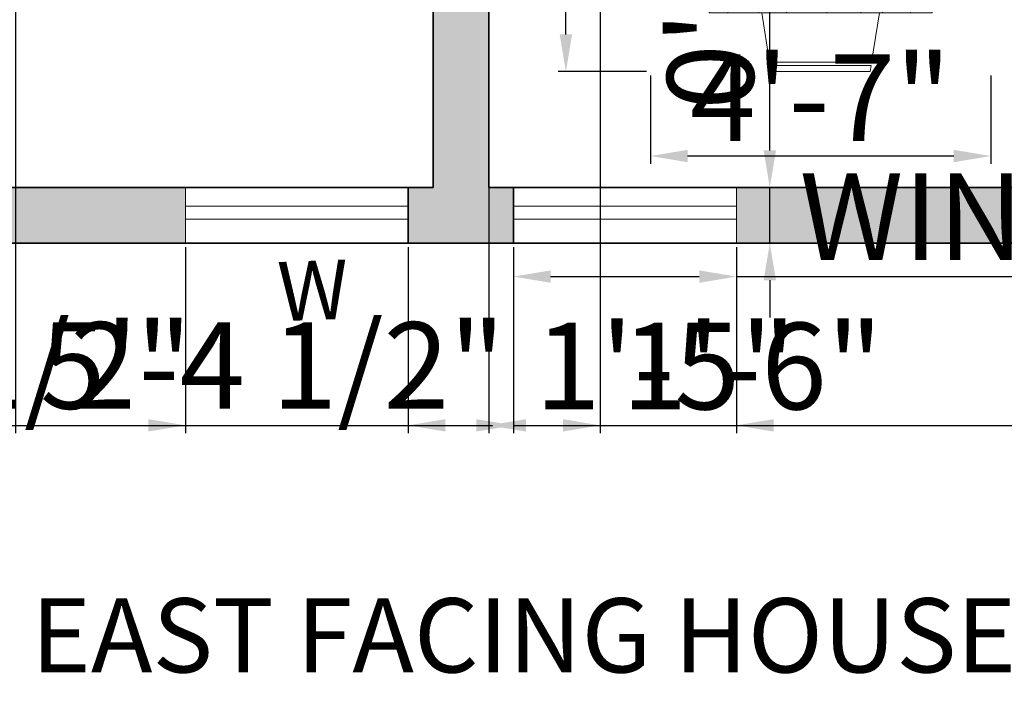
# Model space of a CAD drawing. Units: inches. Extents: x 2961 to 3748, y 1432 to 1961.
# Tile 2 of 9: x 3188 to 3348, y 1432 to 1541. Entities that reach past the tile are written whole.
import ezdxf
from ezdxf.enums import TextEntityAlignment as Align

# ---------------------------------------------------------------- set-up
doc = ezdxf.new("R2010")
doc.units = ezdxf.units.IN
for name, color, linetype, lineweight in [('A-ANNO-DIMS', 2, 'Continuous', 18), ('A-ANNO-TEXT', 7, 'Continuous', 18), ('A-ANNO-TITL', 7, 'Continuous', 25), ('A-FURN', 8, 'Continuous', 18), ('A-GLAZ', 4, 'Continuous', 18), ('A-WALL', 7, 'Continuous', 35), ('A-WALL-PATT', 252, 'Continuous', 13)]:
    doc.layers.add(name, color=color, linetype=linetype, lineweight=lineweight)
doc.styles.get("Standard").update_dxf_attribs({"font": 'arial.ttf'})
doc.dimstyles.new('ISO-25', dxfattribs={"dimtxt": 14, "dimasz": 6, "dimexe": 1.25, "dimexo": 0.625, "dimtad": 1, "dimlunit": 3, "dimtxsty": 'Standard', "dimcen": 2.5, "dimadec": 0, "dimazin": 0, "dimtfac": 1, "dimtmove": 0, "dimatfit": 3, "dimfxl": 1, "dimarcsym": 0})

# ---------------------------------------------------------------- blocks, each defined once
blk = doc.blocks.new('Dining Set - 36 x 72 in.')
for p, q in [((-22, 27.5), (-22.1562, 26.50042)), ((-22, 27.5), (-6, 27.5)), ((-5.8437, 26.49966), (-6, 27.5)), ((6, 27.5), (5.8438, 26.50042)), ((6, 27.5), (22, 27.5)), ((22.1563, 26.49966), (22, 27.5)), ((-22.2343, 26.00059), (-23.4847, 17.99762)), ((-22.2304, 26), (-5.7608, 26)), ((-5.8416, 26.5), (-22.1534, 26.5)), ((-4.5152, 17.99762), (-5.7655, 25.99926)), ((5.7657, 26.00059), (4.5153, 17.99762)), ((5.7696, 26), (22.2392, 26)), ((22.1584, 26.5), (5.8466, 26.5)), ((23.4848, 17.99762), (22.2345, 25.99926)), ((36, 18), (-36, 18)), ((-36, 18), (-36, -18)), ((36, -18), (36, 18)), ((-45.5, 8), (-44.5004, 8.15617)), ((-45.5, 8), (-45.5, -8)), ((-44.5, -8.15843), (-44.5, 8.15338)), ((-44.0006, 8.23428), (-35.9976, 9.48474)), ((-44, 8.23041), (-44, -8.23915)), ((44.0006, 8.23428), (35.9976, 9.48474)), ((44, 8.23041), (44, -8.23915)), ((44.5, -8.15843), (44.5, 8.15338)), ((45.5, 8), (44.5005, 8.15617)), ((45.5, 8), (45.5, -8)), ((-44.4997, -8.15631), (-45.5, -8)), ((-35.9976, -9.48476), (-43.9993, -8.2345)), ((35.9976, -9.48476), (43.9993, -8.2345)), ((44.4997, -8.15631), (45.5, -8)), ((-36, -18), (36, -18)), ((-22.2343, -26.0006), (-23.4847, -17.99762)), ((-4.5152, -17.99762), (-5.7655, -25.99928)), ((5.7657, -26.0006), (4.5153, -17.99762)), ((23.4848, -17.99762), (22.2345, -25.99928)), ((-22.2304, -26), (-5.7608, -26)), ((-22, -27.5), (-22.1562, -26.50044)), ((-5.8416, -26.5), (-22.1534, -26.5)), ((-5.8437, -26.49967), (-6, -27.5)), ((5.7696, -26), (22.2392, -26)), ((6, -27.5), (5.8438, -26.50044)), ((22.1584, -26.5), (5.8466, -26.5)), ((22.1563, -26.49967), (22, -27.5)), ((-22, -27.5), (-6, -27.5)), ((6, -27.5), (22, -27.5))]:
    blk.add_line(p, q)
for points in [[(-36, 15), (-31.1772, 14.97754), (-26.8079, 14.91406), (-22.8538, 14.81543), (-19.276, 14.6875), (-16.0362, 14.53613), (-13.0957, 14.36718), (-10.4159, 14.18652), (-7.9583, 14), (-5.6904, 13.81315), (-3.6035, 13.63021), (-1.6954, 13.45508), (0.0365, 13.29166), (1.5945, 13.14388), (2.9811, 13.01562), (4.1988, 12.9108), (5.25, 12.83333), (6.1393, 12.78613), (6.8802, 12.76823), (7.4883, 12.77767), (7.9792, 12.8125), (8.3685, 12.87077), (8.6719, 12.95052), (8.9049, 13.0498), (9.0833, 13.16666), (9.2205, 13.29899), (9.3216, 13.44401), (9.3895, 13.59879), (9.4271, 13.76041), (9.4373, 13.92594), (9.4232, 14.09245), (9.3875, 14.257), (9.3333, 14.41666), (9.2638, 14.56917), (9.1836, 14.71484), (9.0975, 14.85465), (9.0104, 14.98958), (8.9272, 15.1206), (8.8529, 15.2487), (8.7922, 15.37483), (8.75, 15.5), (8.7305, 15.62467), (8.7344, 15.74739), (8.7617, 15.86621), (8.8125, 15.97916), (8.8867, 16.08431), (8.9844, 16.17968), (9.1055, 16.26334), (9.25, 16.33333), (9.4189, 16.38802), (9.6172, 16.42708), (9.8506, 16.45052), (10.125, 16.45833), (10.4463, 16.45052), (10.8203, 16.42708), (11.2529, 16.38802), (11.75, 16.33333), (12.3184, 16.26318), (12.9694, 16.17838), (13.7151, 16.07991), (14.5677, 15.96875), (15.5395, 15.84586), (16.6426, 15.71224), (17.8893, 15.56884), (19.2917, 15.41666), (20.859, 15.25667), (22.5879, 15.08984), (24.4721, 14.91715), (26.5052, 14.73958), (28.6809, 14.5581), (30.9929, 14.3737), (33.4347, 14.18733), (36, 14)], [(-36, 10), (-28.9766, 10.14274), (-23.1725, 10.20442), (-18.4241, 10.19775), (-14.5677, 10.13541), (-11.4399, 10.03011), (-8.877, 9.89453), (-6.7154, 9.74137), (-4.7917, 9.58333), (-2.9698, 9.43082), (-1.2246, 9.28515), (0.4415, 9.14534), (2.026, 9.01041), (3.5266, 8.87939), (4.9408, 8.7513), (6.266, 8.62516), (7.5, 8.5), (8.6411, 8.37549), (9.6914, 8.2539), (10.6538, 8.13818), (11.5312, 8.03125), (12.3267, 7.93603), (13.043, 7.85547), (13.6831, 7.79248), (14.25, 7.75), (14.7471, 7.7303), (15.1797, 7.73307), (15.5537, 7.75732), (15.875, 7.80208), (16.1494, 7.86637), (16.3828, 7.94922), (16.5811, 8.04964), (16.75, 8.16666), (16.8944, 8.29915), (17.0143, 8.44531), (17.1089, 8.60319), (17.1771, 8.77083), (17.218, 8.94629), (17.2305, 9.1276), (17.2137, 9.31282), (17.1667, 9.5), (17.0895, 9.6875), (16.987, 9.875), (16.8649, 10.0625), (16.7292, 10.25), (16.5856, 10.4375), (16.4401, 10.625), (16.2985, 10.8125), (16.1667, 11), (16.05, 11.18733), (15.9518, 11.3737), (15.8752, 11.5581), (15.8229, 11.73958), (15.798, 11.91715), (15.8034, 12.08984), (15.842, 12.25667), (15.9167, 12.41666), (16.0295, 12.56836), (16.1784, 12.70833), (16.3605, 12.83268), (16.5729, 12.9375), (16.8127, 13.01888), (17.0768, 13.07291), (17.3625, 13.0957), (17.6667, 13.08333), (17.9894, 13.03312), (18.3418, 12.94726), (18.7382, 12.82918), (19.1927, 12.68229), (19.7195, 12.51001), (20.3327, 12.31575), (21.0465, 12.10294), (21.875, 11.875), (22.8357, 11.63354), (23.959, 11.37304), (25.2786, 11.08618), (26.8282, 10.76562), (28.6414, 10.40405), (30.752, 9.99414), (33.1936, 9.52856), (36, 9)], [(-36, 5.5), (-30.7157, 5.3348), (-26.069, 5.20963), (-21.9946, 5.11767), (-18.4271, 5.05208), (-15.3009, 5.00602), (-12.5508, 4.97265), (-10.1112, 4.94515), (-7.9167, 4.91666), (-5.909, 4.88167), (-4.0586, 4.83984), (-2.3429, 4.79215), (-0.7396, 4.73958), (0.7739, 4.6831), (2.22, 4.6237), (3.6213, 4.56233), (5, 4.5), (6.373, 4.43782), (7.7344, 4.3776), (9.0723, 4.32129), (10.375, 4.27083), (11.6309, 4.22819), (12.8281, 4.19531), (13.9551, 4.17415), (15, 4.16666), (15.954, 4.17448), (16.819, 4.19791), (17.6001, 4.23698), (18.3021, 4.29166), (18.9299, 4.36198), (19.4883, 4.44791), (19.9823, 4.54948), (20.4167, 4.66666), (20.7969, 4.79899), (21.1302, 4.94401), (21.4245, 5.09879), (21.6875, 5.26041), (21.9271, 5.42594), (22.1511, 5.59245), (22.3672, 5.757), (22.5834, 5.91666), (22.8065, 6.06868), (23.0404, 6.21093), (23.2879, 6.34147), (23.5521, 6.45833), (23.8358, 6.55957), (24.142, 6.64323), (24.4735, 6.70735), (24.8334, 6.75), (25.2235, 6.76969), (25.642, 6.76692), (26.0858, 6.74267), (26.5521, 6.69791), (27.0379, 6.63362), (27.5404, 6.55078), (28.0565, 6.45036), (28.5834, 6.33333), (29.1242, 6.19987), (29.7071, 6.04687), (30.3661, 5.87044), (31.1354, 5.66666), (32.0493, 5.43164), (33.142, 5.16146), (34.4475, 4.85221), (36, 4.5)], [(-36, -1), (-30.7915, -0.6591), (-26.0195, -0.38216), (-21.6519, -0.16284), (-17.6563, 0.00521), (-14.0005, 0.12833), (-10.6523, 0.21289), (-7.5796, 0.26522), (-4.75, 0.29166), (-2.134, 0.29793), (0.2878, 0.28711), (2.5317, 0.26163), (4.6146, 0.22396), (6.5529, 0.17651), (8.3633, 0.12174), (10.0623, 0.06209), (11.6667, 0), (13.1899, -0.06201), (14.6341, -0.1211), (15.9982, -0.17432), (17.2813, -0.21875), (18.4823, -0.25147), (19.6003, -0.26953), (20.6343, -0.27002), (21.5834, -0.25), (22.4481, -0.20768), (23.2357, -0.14584), (23.9549, -0.06836), (24.6146, 0.02083), (25.2235, 0.11784), (25.7904, 0.21875), (26.3241, 0.31966), (26.8334, 0.41666), (27.3265, 0.50618), (27.8099, 0.58593), (28.2894, 0.65397), (28.7709, 0.70833), (29.2601, 0.74707), (29.763, 0.76823), (30.2855, 0.76985), (30.8334, 0.75), (31.4088, 0.70784), (31.9994, 0.64713), (32.589, 0.57275), (33.1615, 0.48958), (33.7008, 0.4025), (34.1908, 0.3164), (34.6153, 0.23616), (34.9584, 0.16666), (35.2099, 0.11165), (35.3848, 0.07031), (35.504, 0.04069), (35.5886, 0.02083), (35.6594, 0.00879), (35.7377, 0.0026), (35.8442, 0.00032), (36, 0)], [(-36, -6.5), (-27.1843, -6.31267), (-20.084, -6.1263), (-14.469, -5.9419), (-10.1094, -5.76042), (-6.7752, -5.58285), (-4.2363, -5.41016), (-2.2629, -5.24333), (-0.625, -5.08334), (0.8708, -4.93099), (2.2715, -4.78646), (3.5872, -4.64974), (4.8281, -4.52084), (6.0046, -4.39974), (7.127, -4.28646), (8.2053, -4.18099), (9.25, -4.08334), (10.2705, -3.99382), (11.2734, -3.91407), (12.2647, -3.84603), (13.25, -3.79167), (14.2354, -3.75293), (15.2266, -3.73177), (16.2295, -3.73015), (17.25, -3.75), (18.2912, -3.79248), (19.3451, -3.85547), (20.4009, -3.93604), (21.4479, -4.03125), (22.4754, -4.13819), (23.4727, -4.25391), (24.4289, -4.37549), (25.3334, -4.5), (26.1785, -4.62492), (26.9694, -4.74935), (27.7145, -4.87281), (28.4219, -4.99479), (29.1, -5.11483), (29.7572, -5.23242), (30.4016, -5.34709), (31.0417, -5.45834), (31.6837, -5.56437), (32.3262, -5.65821), (32.9658, -5.73153), (33.599, -5.77604), (34.2224, -5.78345), (34.8327, -5.74545), (35.4264, -5.65373), (36, -5.5)], [(-36, -10), (-26.4022, -9.81299), (-18.4675, -9.62891), (-11.9839, -9.45069), (-6.7396, -9.28125), (-2.5226, -9.12354), (0.8789, -8.98047), (3.6769, -8.85498), (6.0833, -8.75), (8.2767, -8.66765), (10.3021, -8.60677), (12.1712, -8.56543), (13.8958, -8.54167), (15.4876, -8.53353), (16.9583, -8.53907), (18.3197, -8.55632), (19.5834, -8.58334), (20.7616, -8.61841), (21.8685, -8.66081), (22.9188, -8.71004), (23.9271, -8.76563), (24.9081, -8.82707), (25.8763, -8.89388), (26.8465, -8.96558), (27.8334, -9.04167), (28.8474, -9.12118), (29.8828, -9.20117), (30.93, -9.27824), (31.9792, -9.34896), (33.0205, -9.40991), (34.0443, -9.45768), (35.0407, -9.48885), (36, -9.5)], [(-36, -14.5), (-30.0881, -14.33513), (-25.0332, -14.21224), (-20.7312, -14.12647), (-17.0781, -14.07292), (-13.97, -14.04671), (-11.3027, -14.04297), (-8.9724, -14.05681), (-6.875, -14.08334), (-4.9224, -14.11833), (-3.0905, -14.16016), (-1.3709, -14.20785), (0.2448, -14.26042), (1.7647, -14.3169), (3.1973, -14.3763), (4.5507, -14.43767), (5.8333, -14.5), (7.0554, -14.5621), (8.235, -14.62175), (9.3922, -14.67652), (10.5469, -14.72396), (11.7192, -14.76164), (12.929, -14.78711), (14.1965, -14.79794), (15.5417, -14.79167), (16.9933, -14.76424), (18.6152, -14.70508), (20.4804, -14.60197), (22.6615, -14.44271), (25.2312, -14.21509), (28.2624, -13.9069), (31.8277, -13.50594), (36, -13)]]:
    blk.add_lwpolyline(points)
blk = doc.blocks.new('WIN-36IN')
for p, q in [((0, 6), (36, 6)), ((0, 3.9), (36, 3.9))]:
    blk.add_line(p, q)
blk.add_lwpolyline([(36, 9), (0, 9), (0, 0), (36, 0)], close=True)
blk = doc.blocks.new('*D20')
at = {"layer": 'A-ANNO-DIMS', "color": 0, "lineweight": -2, "transparency": 16777216}
for p, q in [((3268.27, 1504.01), (3268.27, 1497.99)), ((3304.27, 1504.01), (3304.27, 1497.99)), ((3274.27, 1499.24), (3298.27, 1499.24)), ((3304.27, 1499.24), (3488.68, 1499.24))]:
    blk.add_line(p, q, dxfattribs=at)
at = {"layer": 'A-ANNO-DIMS', "color": 0, "transparency": 16777216}
for points in [[(3274.27, 1500.24), (3274.27, 1498.24), (3268.27, 1499.24)], [(3298.27, 1500.24), (3298.27, 1498.24), (3304.27, 1499.24)]]:
    blk.add_solid(points, dxfattribs=at)
at = {"layer": 'Defpoints', "color": 0, "transparency": 16777216}
for p in [(3268.27, 1504.64), (3304.27, 1504.64), (3304.27, 1499.24)]:
    blk.add_point(p, dxfattribs=at)
at = {"layer": 'A-ANNO-DIMS', "color": 0, "transparency": 16777216, "insert": (3399.47, 1507.11), "char_height": 14, "attachment_point": 5}
blk.add_mtext('WINDOW 3\'-0" TYP.', dxfattribs=at)
blk = doc.blocks.new('*D21')
at = {"layer": 'A-ANNO-DIMS', "color": 0, "lineweight": -2, "transparency": 16777216}
for p, q in [((3309.67, 1519.64), (3309.67, 1612.23)), ((3304.89, 1513.64), (3310.92, 1513.64)), ((3309.67, 1504.64), (3309.67, 1513.64)), ((3304.89, 1504.64), (3310.92, 1504.64)), ((3309.67, 1498.64), (3309.67, 1492.64))]:
    blk.add_line(p, q, dxfattribs=at)
at = {"layer": 'A-ANNO-DIMS', "color": 0, "transparency": 16777216}
for points in [[(3308.67, 1519.64), (3310.67, 1519.64), (3309.67, 1513.64)], [(3308.67, 1498.64), (3310.67, 1498.64), (3309.67, 1504.64)]]:
    blk.add_solid(points, dxfattribs=at)
at = {"layer": 'Defpoints', "color": 0, "transparency": 16777216}
for p in [(3304.27, 1513.64), (3309.67, 1513.64), (3304.27, 1504.64)]:
    blk.add_point(p, dxfattribs=at)
at = {"layer": 'A-ANNO-DIMS', "color": 0, "transparency": 16777216, "insert": (3301.89, 1568.93), "char_height": 14, "attachment_point": 5, "rotation": 90}
blk.add_mtext('0\'-9" TYP.', dxfattribs=at)
blk = doc.blocks.new('*D44')
at = {"layer": 'A-ANNO-DIMS', "color": 0, "lineweight": -2, "transparency": 16777216}
for p, q in [((3276.73, 1623.38), (3276.73, 1784.51)), ((3289.75, 1623.38), (3275.48, 1623.38)), ((3276.73, 1538.38), (3276.73, 1617.38)), ((3289.75, 1532.38), (3275.48, 1532.38))]:
    blk.add_line(p, q, dxfattribs=at)
at = {"layer": 'A-ANNO-DIMS', "color": 0, "transparency": 16777216}
for points in [[(3275.73, 1617.38), (3277.73, 1617.38), (3276.73, 1623.38)], [(3275.73, 1538.38), (3277.73, 1538.38), (3276.73, 1532.38)]]:
    blk.add_solid(points, dxfattribs=at)
at = {"layer": 'Defpoints', "color": 0, "transparency": 16777216}
for p in [(3276.73, 1623.38), (3290.38, 1623.38), (3290.38, 1532.38)]:
    blk.add_point(p, dxfattribs=at)
at = {"layer": 'A-ANNO-DIMS', "color": 0, "transparency": 16777216, "insert": (3268.87, 1706.94), "char_height": 14, "attachment_point": 5, "rotation": 90}
blk.add_mtext('DINING SET 7\'-7"', dxfattribs=at)
blk = doc.blocks.new('*D45')
at = {"layer": 'A-ANNO-DIMS', "color": 0, "lineweight": -2, "transparency": 16777216}
for p, q in [((3290.38, 1531.76), (3290.38, 1517.48)), ((3345.38, 1531.76), (3345.38, 1517.48)), ((3339.38, 1518.73), (3296.38, 1518.73))]:
    blk.add_line(p, q, dxfattribs=at)
at = {"layer": 'A-ANNO-DIMS', "color": 0, "transparency": 16777216}
for points in [[(3296.38, 1519.73), (3296.38, 1517.73), (3290.38, 1518.73)], [(3339.38, 1519.73), (3339.38, 1517.73), (3345.38, 1518.73)]]:
    blk.add_solid(points, dxfattribs=at)
at = {"layer": 'Defpoints', "color": 0, "transparency": 16777216}
for p in [(3290.38, 1532.38), (3345.38, 1532.38), (3290.38, 1518.73)]:
    blk.add_point(p, dxfattribs=at)
at = {"layer": 'A-ANNO-DIMS', "color": 0, "transparency": 16777216, "insert": (3317.88, 1526.36), "char_height": 14, "attachment_point": 5}
blk.add_mtext('4\'-7"', dxfattribs=at)
blk = doc.blocks.new('*D53')
at = {"layer": 'A-ANNO-DIMS', "color": 0, "lineweight": -2, "transparency": 16777216}
for p, q in [((3123.27, 1855.01), (3123.27, 1473.94)), ((3187.8, 1855.01), (3187.8, 1473.94)), ((3129.27, 1475.19), (3181.8, 1475.19)), ((3187.8, 1475.19), (3264.89, 1475.19))]:
    blk.add_line(p, q, dxfattribs=at)
at = {"layer": 'A-ANNO-DIMS', "color": 0, "transparency": 16777216}
for points in [[(3129.27, 1476.19), (3129.27, 1474.19), (3123.27, 1475.19)], [(3181.8, 1476.19), (3181.8, 1474.19), (3187.8, 1475.19)]]:
    blk.add_solid(points, dxfattribs=at)
at = {"layer": 'Defpoints', "color": 0, "transparency": 16777216}
for p in [(3123.27, 1855.64), (3187.8, 1855.64), (3187.8, 1475.19)]:
    blk.add_point(p, dxfattribs=at)
at = {"layer": 'A-ANNO-DIMS', "color": 0, "transparency": 16777216, "insert": (3229.35, 1483.05), "char_height": 14, "attachment_point": 5}
blk.add_mtext('5\'-4 1/2"', dxfattribs=at)
blk = doc.blocks.new('*D56')
at = {"layer": 'A-ANNO-DIMS', "color": 0, "lineweight": -2, "transparency": 16777216}
for p, q in [((3054.27, 1504.01), (3054.27, 1473.94)), ((3215.27, 1504.01), (3215.27, 1473.94)), ((3060.27, 1475.19), (3209.27, 1475.19))]:
    blk.add_line(p, q, dxfattribs=at)
at = {"layer": 'A-ANNO-DIMS', "color": 0, "transparency": 16777216}
for points in [[(3060.27, 1476.19), (3060.27, 1474.19), (3054.27, 1475.19)], [(3209.27, 1476.19), (3209.27, 1474.19), (3215.27, 1475.19)]]:
    blk.add_solid(points, dxfattribs=at)
at = {"layer": 'Defpoints', "color": 0, "transparency": 16777216}
for p in [(3054.27, 1504.64), (3215.27, 1504.64), (3215.27, 1475.19)]:
    blk.add_point(p, dxfattribs=at)
at = {"layer": 'A-ANNO-DIMS', "color": 0, "transparency": 16777216, "insert": (3134.77, 1482.97), "char_height": 14, "attachment_point": 5}
blk.add_mtext('13\'-5"', dxfattribs=at)
blk = doc.blocks.new('*D57')
at = {"layer": 'A-ANNO-DIMS', "color": 0, "lineweight": -2, "transparency": 16777216}
for p, q in [((3251.27, 1504.01), (3251.27, 1473.94)), ((3268.27, 1504.01), (3268.27, 1473.94)), ((3257.27, 1475.19), (3262.27, 1475.19)), ((3268.27, 1475.19), (3311.41, 1475.19))]:
    blk.add_line(p, q, dxfattribs=at)
at = {"layer": 'A-ANNO-DIMS', "color": 0, "transparency": 16777216}
for points in [[(3257.27, 1476.19), (3257.27, 1474.19), (3251.27, 1475.19)], [(3262.27, 1476.19), (3262.27, 1474.19), (3268.27, 1475.19)]]:
    blk.add_solid(points, dxfattribs=at)
at = {"layer": 'Defpoints', "color": 0, "transparency": 16777216}
for p in [(3251.27, 1504.64), (3268.27, 1504.64), (3268.27, 1475.19)]:
    blk.add_point(p, dxfattribs=at)
at = {"layer": 'A-ANNO-DIMS', "color": 0, "transparency": 16777216, "insert": (3292.84, 1482.96), "char_height": 14, "attachment_point": 5}
blk.add_mtext('1\'-5"', dxfattribs=at)
blk = doc.blocks.new('*D58')
at = {"layer": 'A-ANNO-DIMS', "color": 0, "lineweight": -2, "transparency": 16777216}
for p, q in [((3304.27, 1504.01), (3304.27, 1473.94)), ((3456.27, 1504.01), (3456.27, 1473.94)), ((3310.27, 1475.19), (3450.27, 1475.19))]:
    blk.add_line(p, q, dxfattribs=at)
at = {"layer": 'A-ANNO-DIMS', "color": 0, "transparency": 16777216}
for points in [[(3310.27, 1476.19), (3310.27, 1474.19), (3304.27, 1475.19)], [(3450.27, 1476.19), (3450.27, 1474.19), (3456.27, 1475.19)]]:
    blk.add_solid(points, dxfattribs=at)
at = {"layer": 'Defpoints', "color": 0, "transparency": 16777216}
for p in [(3304.27, 1504.64), (3456.27, 1504.64), (3456.27, 1475.19)]:
    blk.add_point(p, dxfattribs=at)
at = {"layer": 'A-ANNO-DIMS', "color": 0, "transparency": 16777216, "insert": (3380.27, 1482.96), "char_height": 14, "attachment_point": 5}
blk.add_mtext('12\'-8"', dxfattribs=at)
blk = doc.blocks.new('*D77')
at = {"layer": 'A-ANNO-DIMS', "color": 0, "lineweight": -2, "transparency": 16777216}
for p, q in [((3264.27, 1775.91), (3264.27, 1473.94)), ((3282.27, 1775.91), (3282.27, 1473.94)), ((3270.27, 1475.19), (3276.27, 1475.19)), ((3282.27, 1475.19), (3325.41, 1475.19))]:
    blk.add_line(p, q, dxfattribs=at)
at = {"layer": 'A-ANNO-DIMS', "color": 0, "transparency": 16777216}
for points in [[(3270.27, 1476.19), (3270.27, 1474.19), (3264.27, 1475.19)], [(3276.27, 1476.19), (3276.27, 1474.19), (3282.27, 1475.19)]]:
    blk.add_solid(points, dxfattribs=at)
at = {"layer": 'Defpoints', "color": 0, "transparency": 16777216}
for p in [(3264.27, 1776.53), (3282.27, 1776.53), (3282.27, 1475.19)]:
    blk.add_point(p, dxfattribs=at)
at = {"layer": 'A-ANNO-DIMS', "color": 0, "transparency": 16777216, "insert": (3306.84, 1482.96), "char_height": 14, "attachment_point": 5}
blk.add_mtext('1\'-6"', dxfattribs=at)
blk = doc.blocks.new('*D84')
at = {"layer": 'A-ANNO-DIMS', "color": 0, "lineweight": -2, "transparency": 16777216}
for p, q in [((3123.27, 1855.01), (3123.27, 1473.94)), ((3137.88, 1855.01), (3137.88, 1473.94)), ((3129.27, 1475.19), (3131.88, 1475.19)), ((3137.88, 1475.19), (3213.65, 1475.19))]:
    blk.add_line(p, q, dxfattribs=at)
at = {"layer": 'A-ANNO-DIMS', "color": 0, "transparency": 16777216}
for points in [[(3129.27, 1476.19), (3129.27, 1474.19), (3123.27, 1475.19)], [(3131.88, 1476.19), (3131.88, 1474.19), (3137.88, 1475.19)]]:
    blk.add_solid(points, dxfattribs=at)
at = {"layer": 'Defpoints', "color": 0, "transparency": 16777216}
for p in [(3123.27, 1855.64), (3137.88, 1855.64), (3137.88, 1475.19)]:
    blk.add_point(p, dxfattribs=at)
at = {"layer": 'A-ANNO-DIMS', "color": 0, "transparency": 16777216, "insert": (3178.76, 1483.05), "char_height": 14, "attachment_point": 5}
blk.add_mtext('1\'-2 1/2"', dxfattribs=at)

msp = doc.modelspace()

# ---------------------------------------------------------------- hatches: boundary and pattern name
at = {"layer": 'A-WALL-PATT'}
h = msp.add_hatch(color=256, dxfattribs=at)
h.set_gradient(color1=(41, 49, 137), color2=(41, 49, 137), tint=1)
h.paths.add_polyline_path([(3255.267, 1671.639), (3255.267, 1513.639), (3251.267, 1513.639), (3251.267, 1504.639), (3268.267, 1504.639), (3268.267, 1513.639), (3264.267, 1513.639), (3264.267, 1671.639), (3259.767, 1671.639)])
h.paths.add_polyline_path([(3063.267, 1513.639), (3063.267, 1677.639), (3054.267, 1677.639), (3054.267, 1504.639), (3215.267, 1504.639), (3215.267, 1513.639)])
h.paths.add_polyline_path([(3304.267, 1513.639), (3304.267, 1504.639), (3456.267, 1504.639), (3456.267, 1513.639), (3390.267, 1513.639), (3390.267, 1605.639), (3384.267, 1605.639), (3384.267, 1513.639)])
h.paths.add_polyline_path([(3510.267, 1605.639), (3510.267, 1513.639), (3492.267, 1513.639), (3492.267, 1504.639), (3546.267, 1504.639), (3546.267, 1513.639), (3519.267, 1513.639), (3519.267, 1605.639)])
h.paths.add_polyline_path([(3340.267, 1654.639), (3340.267, 1645.639), (3510.267, 1645.639), (3510.267, 1641.639), (3519.267, 1641.639), (3519.267, 1658.639), (3510.267, 1658.639), (3510.267, 1654.639)])
h.paths.add_polyline_path([(3223.801, 1864.639), (3223.801, 1855.639), (3255.267, 1855.639), (3255.267, 1772.534), (3264.267, 1772.534), (3264.267, 1855.639), (3303.267, 1855.639), (3303.267, 1864.639)])
h.paths.add_polyline_path([(3339.267, 1864.639), (3339.267, 1855.639), (3435.267, 1855.639), (3435.267, 1864.639)])
h.paths.add_polyline_path([(3471.267, 1864.639), (3471.267, 1855.639), (3510.267, 1855.639), (3510.267, 1827.639), (3519.267, 1827.639), (3519.267, 1864.639)])
h.paths.add_polyline_path([(3510.267, 1767.639), (3510.267, 1739.639), (3519.267, 1739.639), (3519.267, 1767.639)])
h.paths.add_polyline_path([(3123.267, 1726.639), (3123.267, 1855.639), (3187.801, 1855.639), (3187.801, 1864.639), (3054.267, 1864.639), (3054.267, 1837.201), (3063.267, 1837.201), (3063.267, 1855.639), (3117.267, 1855.639), (3117.267, 1726.639), (3103.267, 1726.639), (3103.267, 1717.639), (3255.267, 1717.639), (3255.267, 1713.639), (3264.267, 1713.639), (3264.267, 1730.534), (3255.267, 1730.639), (3255.267, 1726.639)])
h.paths.add_polyline_path([(3597.267, 1654.639), (3597.267, 1513.639), (3570.267, 1513.639), (3570.267, 1504.639), (3603.267, 1504.639), (3603.267, 1654.639)])
h.paths.add_polyline_path([(3054.267, 1813.201), (3054.267, 1713.639), (3063.267, 1713.639), (3063.267, 1717.639), (3069.267, 1717.639), (3069.267, 1726.639), (3063.267, 1726.639), (3063.267, 1813.201)], flags=17)

# ---------------------------------------------------------------- linework, layer by layer
at = {"layer": 'A-WALL'}
for p, q in [((3264.267, 1513.639), (3264.267, 1855.639)), ((3255.267, 1513.639), (3255.267, 1671.639)), ((3255.267, 1513.639), (3063.267, 1513.639)), ((3251.267, 1513.639), (3251.267, 1504.639)), ((3384.267, 1513.639), (3264.267, 1513.639)), ((3268.267, 1513.639), (3268.267, 1504.639)), ((3603.267, 1504.639), (3054.267, 1504.639))]:
    msp.add_line(p, q, dxfattribs=at)

# ---------------------------------------------------------------- block references
at = {"layer": 'A-FURN', "rotation": 90}
msp.add_blockref('Dining Set - 36 x 72 in.', (3317.88, 1577.882), dxfattribs=at)
at = {"layer": 'A-GLAZ'}
for p in [(3215.267, 1504.639), (3268.267, 1504.639)]:
    msp.add_blockref('WIN-36IN', p, dxfattribs=at)

# ---------------------------------------------------------------- texts
at = {"layer": 'A-ANNO-TEXT'}
msp.add_text('W', height=9.571, rotation=2.15165, dxfattribs=at).set_placement((3236.067, 1492.227), align=Align.CENTER)
at = {"layer": 'A-ANNO-TITL'}
msp.add_text('EAST FACING HOUSE PLAN (45\'9"X30\')', height=12, dxfattribs=at).set_placement((3335.479, 1435.239), align=Align.CENTER)

# ---------------------------------------------------------------- dimensions: what is measured, and where the dimension line sits
at = {"layer": 'A-ANNO-DIMS'}
for base, p1, p2, picture, middle in [((3187.801, 1475.189), (3123.267, 1855.639), (3187.801, 1855.639), '*D53', (3229.345, 1483.052)), ((3137.877, 1475.189), (3123.267, 1855.639), (3137.877, 1855.639), '*D84', (3178.762, 1483.052)), ((3282.267, 1475.189), (3264.267, 1776.534), (3282.267, 1776.534), '*D77', (3306.841, 1482.962)), ((3215.267, 1475.189), (3054.267, 1504.639), (3215.267, 1504.639), '*D56', (3134.767, 1482.966)), ((3268.267, 1475.189), (3251.267, 1504.639), (3268.267, 1504.639), '*D57', (3292.841, 1482.962)), ((3456.267, 1475.189), (3304.267, 1504.639), (3456.267, 1504.639), '*D58', (3380.267, 1482.962))]:
    dim = msp.add_linear_dim(base=base, p1=p1, p2=p2, dimstyle='ISO-25', override={"dimdec": 1, "dimlfac": 1, "dimrnd": 0, "dimzin": 1, "dimdsep": 46, "dimlunit": 4, "dimfrac": 2}, dxfattribs=at)
    dim.commit()
    dim.dimension.update_dxf_attribs({"geometry": picture, "text_midpoint": middle})
for base, p1, p2, text, picture, middle in [((3276.73, 1623.382), (3290.38, 1532.382), (3290.38, 1623.382), 'DINING SET <>', '*D44', (3268.866, 1706.945)), ((3309.667, 1513.639), (3304.267, 1504.639), (3304.267, 1513.639), '<> TYP.', '*D21', (3301.894, 1568.932))]:
    dim = msp.add_linear_dim(base=base, p1=p1, p2=p2, angle=90, text=text, dimstyle='ISO-25', override={"dimdec": 1, "dimlfac": 1, "dimrnd": 0, "dimzin": 1, "dimdsep": 46, "dimlunit": 4, "dimfrac": 2}, dxfattribs=at)
    dim.commit()
    dim.dimension.update_dxf_attribs({"geometry": picture, "text_midpoint": middle})
dim = msp.add_linear_dim(base=(3304.267, 1499.239), p1=(3268.267, 1504.639), p2=(3304.267, 1504.639), text='WINDOW <> TYP.', dimstyle='ISO-25', override={"dimdec": 1, "dimlfac": 1, "dimrnd": 0, "dimzin": 1, "dimdsep": 46, "dimlunit": 4, "dimfrac": 2}, dxfattribs=at)
dim.commit()
dim.dimension.update_dxf_attribs({"geometry": '*D20', "text_midpoint": (3399.471, 1507.112)})
dim = msp.add_linear_dim(base=(3290.38, 1518.732), p1=(3345.38, 1532.382), p2=(3290.38, 1532.382), angle=180, dimstyle='ISO-25', override={"dimdec": 1, "dimlfac": 1, "dimrnd": 0, "dimzin": 1, "dimdsep": 46, "dimlunit": 4, "dimfrac": 2}, dxfattribs=at)
dim.commit()
dim.dimension.update_dxf_attribs({"geometry": '*D45', "text_midpoint": (3317.88, 1526.357)})

doc.saveas('drawing.dxf')
